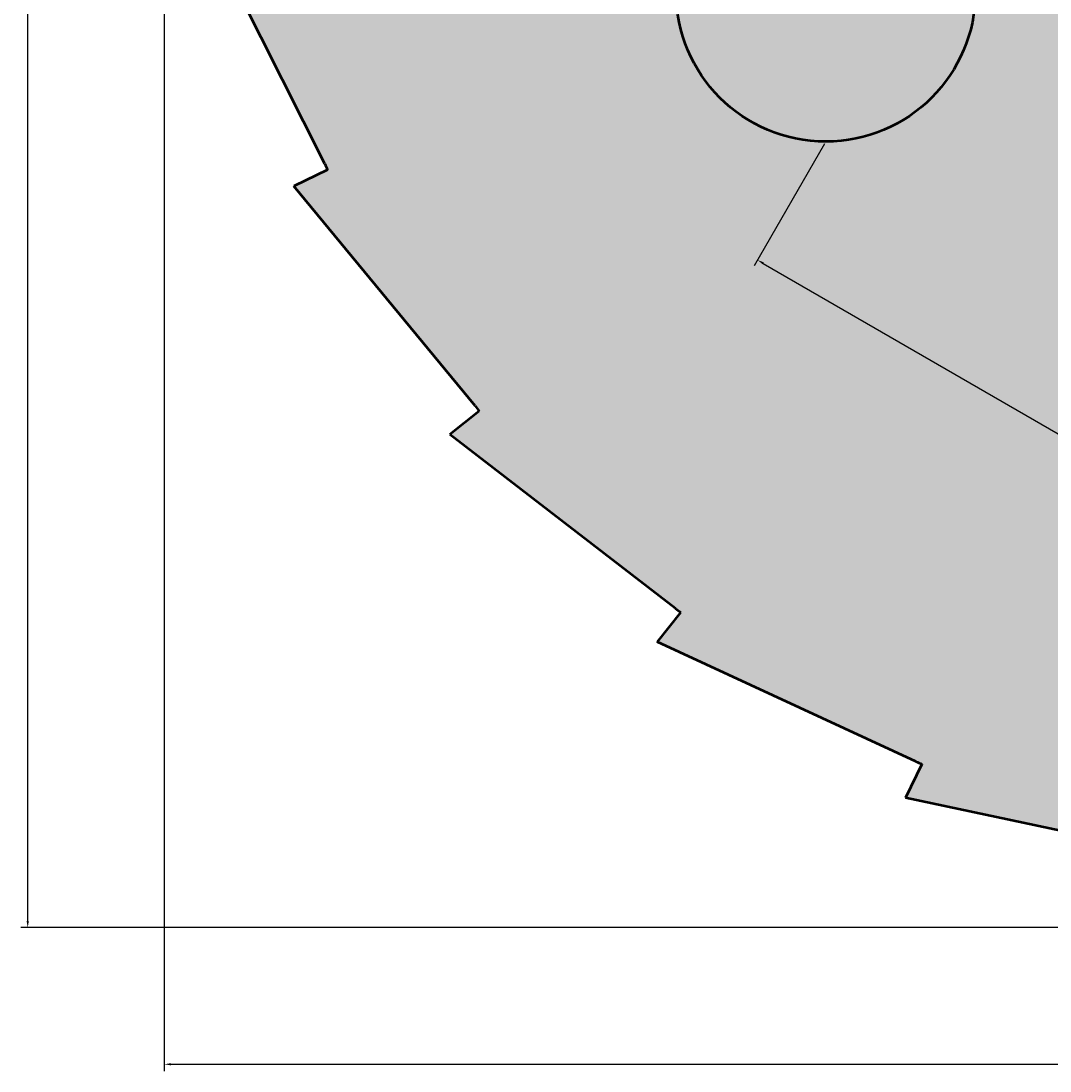
# Model space of a CAD drawing. Units: millimetres. Extents: x 2943.6 to 3032.7, y 1562 to 1639.7.
# Tile 1 of 9: x 2943.6 to 2971.1, y 1562 to 1590.1. Entities that reach past the tile are written whole.
import ezdxf

# ---------------------------------------------------------------- set-up
doc = ezdxf.new("R2010")
doc.units = ezdxf.units.MM
doc.layers.add('M-DIMS', color=2, linetype='Continuous', lineweight=18)
doc.layers.add('M-OUTL', color=7, linetype='Continuous', lineweight=50)
doc.layers.add('M-HATC', color=7, linetype='Continuous', lineweight=18, true_color=0xffffff)
doc.styles.get("Standard").update_dxf_attribs({"font": 'arial.ttf'})
doc.dimstyles.get("Standard").update_dxf_attribs({"dimtxt": 0.18, "dimasz": 0.18, "dimexe": 0.18, "dimexo": 0.0625, "dimgap": 0.09, "dimtad": 0, "dimtih": 1, "dimtoh": 1, "dimdec": 4, "dimzin": 0, "dimdsep": 46, "dimtxsty": 'Standard', "dimcen": 0.09, "dimadec": 0, "dimazin": 0, "dimtfac": 1, "dimtdec": 4, "dimtofl": 0, "dimtmove": 0, "dimatfit": 3, "dimfxl": 1, "dimtolj": 1, "dimtzin": 0, "dimarcsym": 0})

# ---------------------------------------------------------------- blocks, each defined once
blk = doc.blocks.new('*U1')
blk.add_circle((0, 0), 4)
blk = doc.blocks.new('*U2')
at = {"layer": 'M-OUTL', "color": 0, "linetype": 'ByBlock', "lineweight": -2, "transparency": 16777216, "rotation": 120}
blk.add_blockref('*U1', (2965.149, 1590.848), dxfattribs=at)
blk = doc.blocks.new('*D3')
at = {"layer": 'Defpoints', "color": 0, "transparency": 16777216}
for p in [(2947.469, 1600.848), (3017.469, 1600.848), (3017.469, 1562.198)]:
    blk.add_point(p, dxfattribs=at)
at = {"layer": 'M-DIMS', "color": 0, "lineweight": -2, "transparency": 16777216}
for p, q in [((2947.469, 1600.786), (2947.469, 1562.018)), ((3017.469, 1600.786), (3017.469, 1562.018)), ((2947.649, 1562.198), (2982.251, 1562.198)), ((3017.289, 1562.198), (2982.687, 1562.198))]:
    blk.add_line(p, q, dxfattribs=at)
at = {"layer": 'M-DIMS', "color": 0, "transparency": 16777216}
for points in [[(2947.649, 1562.228), (2947.649, 1562.168), (2947.469, 1562.198)], [(3017.289, 1562.228), (3017.289, 1562.168), (3017.469, 1562.198)]]:
    blk.add_solid(points, dxfattribs=at)
at = {"layer": 'M-DIMS', "color": 0, "transparency": 16777216, "insert": (2982.469, 1562.198), "char_height": 0.18, "attachment_point": 5}
blk.add_mtext('\\A1;70', dxfattribs=at)
blk = doc.blocks.new('*D4')
at = {"layer": 'Defpoints', "color": 0, "transparency": 16777216}
for p in [(2943.819, 1635.848), (2982.469, 1635.848), (2982.469, 1565.848)]:
    blk.add_point(p, dxfattribs=at)
at = {"layer": 'M-DIMS', "color": 0, "lineweight": -2, "transparency": 16777216}
for p, q in [((2982.407, 1635.848), (2943.639, 1635.848)), ((2943.819, 1635.668), (2943.819, 1601.03)), ((2943.819, 1566.028), (2943.819, 1600.666)), ((2982.407, 1565.848), (2943.639, 1565.848))]:
    blk.add_line(p, q, dxfattribs=at)
at = {"layer": 'M-DIMS', "color": 0, "transparency": 16777216}
for points in [[(2943.789, 1635.668), (2943.849, 1635.668), (2943.819, 1635.848)], [(2943.789, 1566.028), (2943.849, 1566.028), (2943.819, 1565.848)]]:
    blk.add_solid(points, dxfattribs=at)
at = {"layer": 'M-DIMS', "color": 0, "transparency": 16777216, "insert": (2943.819, 1600.848), "char_height": 0.18, "attachment_point": 5}
blk.add_mtext('\\A1;70', dxfattribs=at)
blk = doc.blocks.new('*D6')
at = {"layer": 'Defpoints', "color": 0, "transparency": 16777216}
for p in [(2965.149, 1586.848), (2963.324, 1583.687), (2982.469, 1576.848)]:
    blk.add_point(p, dxfattribs=at)
at = {"layer": 'M-DIMS', "color": 0, "lineweight": -2, "transparency": 16777216}
for p, q in [((2965.118, 1586.794), (2963.234, 1583.531)), ((2963.48, 1583.597), (2971.764, 1578.814)), ((2980.488, 1573.777), (2972.204, 1578.56)), ((2982.438, 1576.794), (2980.554, 1573.531))]:
    blk.add_line(p, q, dxfattribs=at)
at = {"layer": 'M-DIMS', "color": 0, "transparency": 16777216}
for points in [[(2963.495, 1583.623), (2963.465, 1583.571), (2963.324, 1583.687)], [(2980.503, 1573.803), (2980.473, 1573.751), (2980.644, 1573.687)]]:
    blk.add_solid(points, dxfattribs=at)
at = {"layer": 'M-DIMS', "color": 0, "transparency": 16777216, "insert": (2971.984, 1578.687), "char_height": 0.18, "attachment_point": 5}
blk.add_mtext('\\A1;20', dxfattribs=at)

msp = doc.modelspace()

# ---------------------------------------------------------------- hatches: boundary and pattern name
at = {"layer": 'M-HATC'}
h = msp.add_hatch(color=256, dxfattribs=at)
h.set_gradient(color1=(0, 0, 255), color2=(255, 255, 0), tint=1, name='INVCURVED')
h.paths.add_polyline_path([(2949.361, 1608.583, 0.001279), (2949.322, 1608.414), (2948.347, 1608.637), (2948.473, 1600.848), (2947.469, 1600.848), (2949.283, 1593.452, 0.001279), (2949.322, 1593.283), (2948.347, 1593.06), (2951.761, 1586.253, 0.001279), (2951.836, 1586.096), (2950.935, 1585.662), (2955.779, 1579.786, 0.001279), (2955.887, 1579.65), (2955.105, 1579.026), (2961.135, 1574.375, 0.001279), (2961.271, 1574.266), (2960.647, 1573.484), (2967.561, 1570.291, 0.001279), (2967.717, 1570.215), (2967.283, 1569.314), (2974.734, 1567.74, 0.001279), (2974.904, 1567.701), (2974.681, 1566.726), (2982.295, 1566.849, 0.001279), (2982.469, 1566.848), (2982.469, 1565.848), (2989.865, 1567.662, 0.001279), (2990.035, 1567.701), (2990.258, 1566.726), (2997.064, 1570.14, 0.001279), (2997.221, 1570.215), (2997.655, 1569.314), (3003.532, 1574.158, 0.001279), (3003.668, 1574.266), (3004.291, 1573.484), (3008.943, 1579.514, 0.001279), (3009.052, 1579.65), (3009.833, 1579.026), (3013.026, 1585.94, 0.001279), (3013.102, 1586.096), (3014.003, 1585.662), (3015.578, 1593.113, 0.001279), (3015.617, 1593.283), (3016.592, 1593.06), (3016.469, 1600.674, 0.001279), (3016.469, 1600.848), (3017.469, 1600.848), (3015.655, 1608.244, 0.001279), (3015.617, 1608.414), (3016.592, 1608.637), (3013.177, 1615.443, 0.001279), (3013.102, 1615.6), (3014.003, 1616.034), (3009.16, 1621.911, 0.001279), (3009.052, 1622.047), (3009.833, 1622.67), (3003.804, 1627.322, 0.001279), (3003.668, 1627.431), (3004.291, 1628.212), (2997.378, 1631.405, 0.001279), (2997.221, 1631.481), (2997.655, 1632.382), (2990.204, 1633.957, 0.001279), (2990.035, 1633.996), (2990.258, 1634.971), (2982.469, 1634.845), (2982.469, 1635.848), (2975.073, 1634.034, 0.001279), (2974.904, 1633.996), (2974.681, 1634.971), (2967.874, 1631.556, 0.001279), (2967.717, 1631.481), (2967.283, 1632.382), (2961.407, 1627.539, 0.001279), (2961.271, 1627.431), (2960.647, 1628.212), (2955.996, 1622.183, 0.001279), (2955.887, 1622.047), (2955.105, 1622.67), (2951.912, 1615.757, 0.001279), (2951.836, 1615.6), (2950.935, 1616.034)])
h.paths.add_polyline_path([(2969.149, 1610.848, -1), (2961.149, 1610.848, -1)], flags=16)
h.paths.add_polyline_path([(2969.149, 1590.848, -1), (2961.149, 1590.848, -1)], flags=16)
h.paths.add_polyline_path([(2992.469, 1600.848, -1), (2972.469, 1600.848, -1)], flags=16)
h.paths.add_polyline_path([(2978.469, 1620.848, -1), (2986.469, 1620.848, -1)], flags=16)
h.paths.add_polyline_path([(2981.469, 1605.236), (2981.469, 1606.848), (2983.469, 1606.848), (2983.469, 1605.236, -8.887482)], flags=0)
h.paths.add_polyline_path([(2986.469, 1580.848, -1), (2978.469, 1580.848, -1)], flags=16)
h.paths.add_polyline_path([(3003.79, 1610.848, -1), (2995.79, 1610.848, -1)], flags=16)
h.paths.add_polyline_path([(3003.79, 1590.848, -1), (2995.79, 1590.848, -1)], flags=16)
h = msp.add_hatch(color=256, dxfattribs=at)
h.paths.add_polyline_path([(2978.469, 1620.848, 1), (2986.469, 1620.848, 1)])
h.paths.add_polyline_path([(2995.79, 1610.848, 1), (3003.79, 1610.848, 1)])
h.paths.add_polyline_path([(3003.79, 1590.848, 1), (2995.79, 1590.848, 1)])
h.paths.add_polyline_path([(2986.469, 1580.848, 1), (2978.469, 1580.848, 1)])
h.paths.add_polyline_path([(2969.149, 1590.848, 1), (2961.149, 1590.848, 1)])
h.paths.add_polyline_path([(2961.149, 1610.848, 1), (2969.149, 1610.848, 1)])

# ---------------------------------------------------------------- linework, layer by layer
at = {"layer": 'M-OUTL'}
for p, q in [((2951.761, 1586.253), (2948.347, 1593.06)), ((2951.836, 1586.096), (2950.935, 1585.662)), ((2955.779, 1579.786), (2950.935, 1585.662)), ((2955.887, 1579.65), (2955.105, 1579.026)), ((2961.135, 1574.375), (2955.105, 1579.026)), ((2961.271, 1574.266), (2960.647, 1573.484)), ((2967.561, 1570.291), (2960.647, 1573.484)), ((2967.717, 1570.215), (2967.283, 1569.314)), ((2974.734, 1567.74), (2967.283, 1569.314))]:
    msp.add_line(p, q, dxfattribs=at)
for start, end in [(205.4212, 205.7143), (218.2783, 218.5714), (231.1355, 231.4286), (243.9926, 244.2857)]:
    msp.add_arc((2982.469, 1600.848), 34, start, end, dxfattribs=at)

# ---------------------------------------------------------------- block references
msp.add_blockref('*U2', (0, 0), dxfattribs=at)

# ---------------------------------------------------------------- dimensions: what is measured, and where the dimension line sits
at = {"layer": 'M-DIMS'}
for base, p1, p2, angle, picture, middle in [((2943.819, 1635.848), (2982.469, 1565.848), (2982.469, 1635.848), 90, '*D4', (2943.819, 1600.848)), ((2963.324, 1583.687), (2982.469, 1576.848), (2965.149, 1586.848), 150, '*D6', (2971.984, 1578.687))]:
    dim = msp.add_linear_dim(base=base, p1=p1, p2=p2, angle=angle, dimstyle='Standard', override={"dimdec": 0, "dimlfac": 1, "dimrnd": 0, "dimzin": 0, "dimdsep": 46, "dimlunit": 2}, dxfattribs=at)
    dim.commit()
    dim.dimension.update_dxf_attribs({"geometry": picture, "text_midpoint": middle})
dim = msp.add_linear_dim(base=(3017.469, 1562.198), p1=(2947.469, 1600.848), p2=(3017.469, 1600.848), dimstyle='Standard', override={"dimdec": 0, "dimlfac": 1, "dimrnd": 0, "dimzin": 0, "dimdsep": 46, "dimlunit": 2}, dxfattribs=at)
dim.commit()
dim.dimension.update_dxf_attribs({"geometry": '*D3', "text_midpoint": (2982.469, 1562.198)})

doc.saveas('drawing.dxf')
